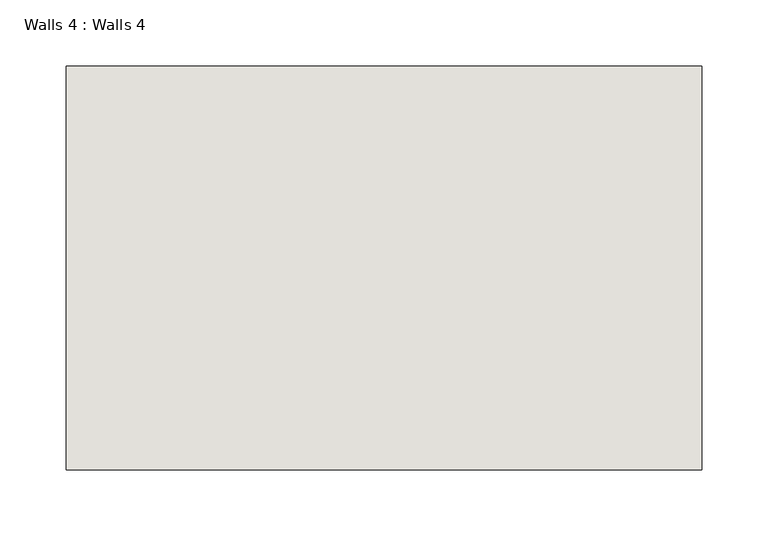
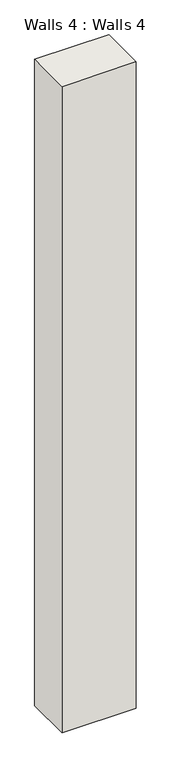
"""IFC4 building model written with IfcOpenShell, lengths in millimetres: wall geometry, Walls 4 : Walls 4."""

from ifc_helpers import new_model, si_unit, frame, origin, place, context, project, spatial, polyline, outline, extrude, source, transform, mapped, element, save


def walls_4_walls_4_9e78723f(model_context):
    return source(origin(), model_context, "Body", "SweptSolid", [
        extrude(outline(polyline([(-4755.1093643, 1328.1827135), (-5234.779577, 1328.1827135), (-5234.779577, 1632.9827135), (-4755.1093643, 1632.9827135), (-4755.1093643, 1328.1827135)])), frame((0.0, 0.0, 4484.7757388), z_axis=(0.0, 0.0, 1.0), x_axis=(1.0, 0.0, 0.0)), (0.0, 0.0, 1.0), 4419.6),
    ])


if __name__ == "__main__":
    model = new_model("IFC4")
    model_context = context("Model", 3, world=origin())
    ifc_project = project(units=[si_unit("LENGTHUNIT", "METRE", prefix="MILLI")], contexts=[model_context])
    site = spatial("IfcSite", under=ifc_project)
    building = spatial("IfcBuilding", under=site)
    placement = place(None, origin())
    walls_4_walls_4_shape = walls_4_walls_4_9e78723f(model_context)
    element("IfcWall", 1, ObjectType="Walls 4 : Walls 4", at=placement, inside=building, context=model_context, shape_type="MappedRepresentation", body=[
        mapped(walls_4_walls_4_shape, transform((0.0, 0.0, 0.0), x_axis=(1.0, 0.0, 0.0), y_axis=(0.0, 1.0, 0.0), z_axis=(0.0, 0.0, 1.0))),
    ])
    save(model, "model.ifc")

# Revit data of these elements
# Element 1 (IfcWall, "Walls 4 : Walls 4")
#   Materials on its faces: "Default Wall"
# Materials
#   "Default Wall": colour RGB 128 128 128, transparency 0
